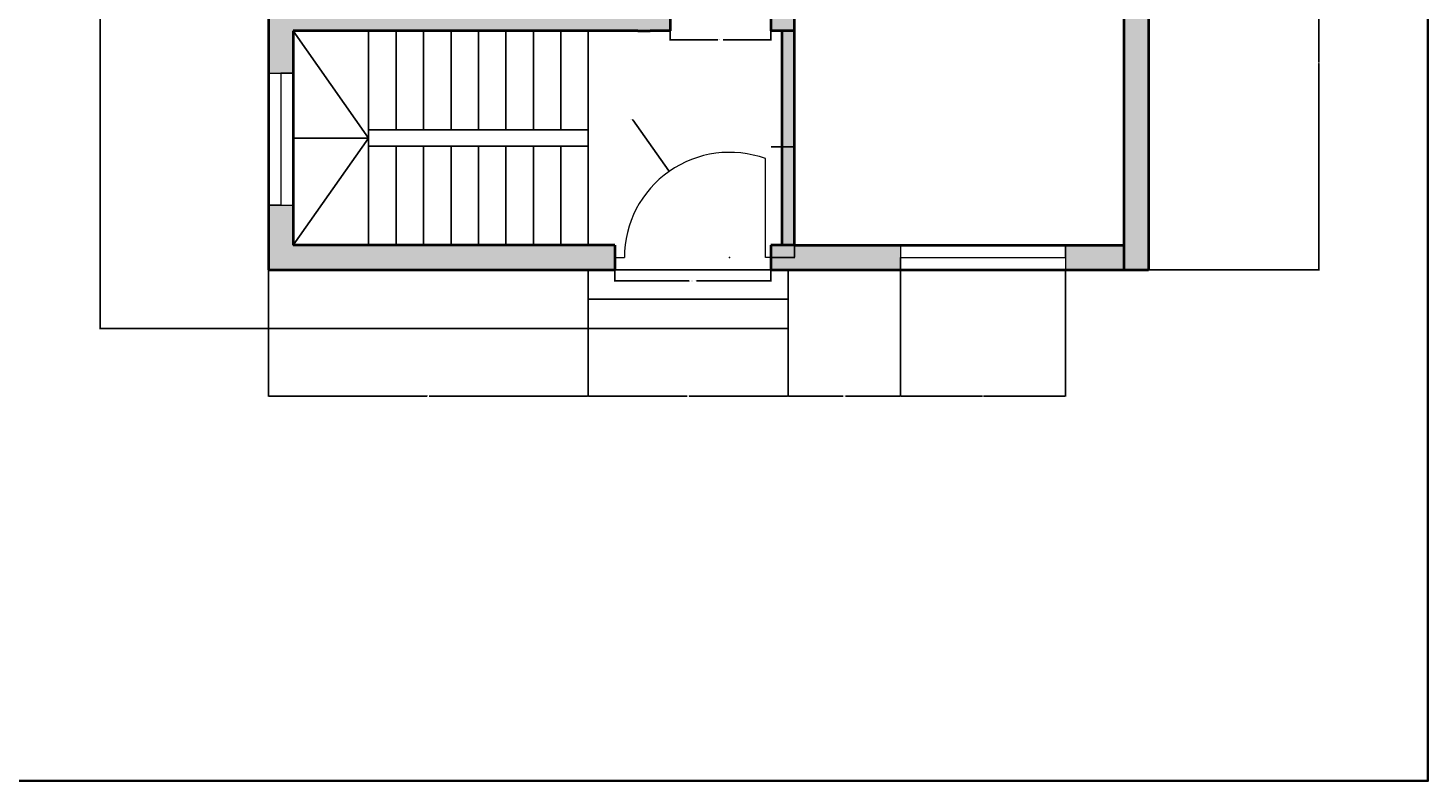
# Model space of a CAD drawing. Units: inches. Extents: x 1441 to 2460, y 1648 to 2683.
# Tile 30 of 35: x 1950 to 2460, y 1648 to 1922. Entities that reach past the tile are written whole.
import ezdxf

# ---------------------------------------------------------------- set-up
doc = ezdxf.new("R2010")
doc.units = ezdxf.units.IN
for name, color, linetype, lineweight in [('A-ANNO-DIMS', 2, 'Continuous', 18), ('A-ANNO-TTLB', 7, 'Continuous', 35), ('A-DOOR', 3, 'Continuous', 20), ('A-FLOR-STRS', 7, 'Continuous', 25), ('A-GLAZ', 4, 'Continuous', 18), ('A-WALL', 7, 'Continuous', 40)]:
    doc.layers.add(name, color=color, linetype=linetype, lineweight=lineweight)
doc.layers.add('A-WALL-PATT', color=251, linetype='Continuous', lineweight=13, true_color=0x636466)
doc.styles.get("Standard").update_dxf_attribs({"font": 'arial.ttf'})
doc.dimstyles.get("Standard").update_dxf_attribs({"dimtxt": 0.18, "dimasz": 0.18, "dimexe": 0.18, "dimexo": 0.0625, "dimgap": 0.09, "dimtad": 0, "dimtih": 1, "dimtoh": 1, "dimdec": 4, "dimzin": 0, "dimdsep": 46, "dimtxsty": 'Standard', "dimcen": 0.09, "dimadec": 0, "dimazin": 0, "dimtfac": 1, "dimtdec": 4, "dimtofl": 0, "dimtmove": 0, "dimatfit": 3, "dimfxl": 1, "dimtolj": 1, "dimtzin": 0, "dimarcsym": 0})

# ---------------------------------------------------------------- blocks, each defined once
blk = doc.blocks.new('DOOR-ENTRY-OUTER')
for p, q in [((54.89, 0), (54.89, 36)), ((0, 0), (1.52, 0)), ((1.52, 0), (3.52, 0)), ((56.89, 0), (54.89, 0))]:
    blk.add_line(p, q)
blk.add_arc((41.82, 0), 38.3, 70.0399, 180)
blk = doc.blocks.new('WIN-48-SASH')
for p, q in [((9, 48), (4.5, 48)), ((4.5, 48), (4.5, 0)), ((4.5, 0), (0, 0))]:
    blk.add_line(p, q)
blk = doc.blocks.new('STAIR-RETURN-PLAN')
for p, q in [((27.5, 39), (0, 78)), ((27.5, 0), (27.5, 78)), ((37.5, 42), (37.5, 78)), ((47.5, 42), (47.5, 78)), ((57.5, 42), (57.5, 78)), ((67.5, 42), (67.5, 78)), ((77.5, 42), (77.5, 78)), ((87.5, 42), (87.5, 78)), ((97.5, 42), (97.5, 78)), ((107.5, 0), (107.5, 78)), ((107.5, 42), (27.5, 42)), ((27.5, 39), (0, 39)), ((0, 39), (27.5, 39)), ((27.5, 39), (0, 0)), ((107.5, 36), (27.5, 36)), ((37.5, 0), (37.5, 36)), ((47.5, 0), (47.5, 36)), ((57.5, 0), (57.5, 36)), ((67.5, 0), (67.5, 36)), ((77.5, 0), (77.5, 36)), ((87.5, 0), (87.5, 36)), ((97.5, 0), (97.5, 36))]:
    blk.add_line(p, q)
blk = doc.blocks.new('*D54')
at = {"layer": 'A-ANNO-DIMS', "color": 0, "lineweight": -2, "transparency": 16777216}
for p, q in [((2164.02, 1838.63), (2164.02, 1829.98)), ((2220.91, 1838.63), (2220.91, 1829.98)), ((2164.2, 1830.16), (2191.07, 1830.16)), ((2220.73, 1830.16), (2193.86, 1830.16))]:
    blk.add_line(p, q, dxfattribs=at)
at = {"layer": 'A-ANNO-DIMS', "color": 0, "transparency": 16777216}
for points in [[(2164.2, 1830.19), (2164.2, 1830.13), (2164.02, 1830.16)], [(2220.73, 1830.19), (2220.73, 1830.13), (2220.91, 1830.16)]]:
    blk.add_solid(points, dxfattribs=at)
at = {"layer": 'Defpoints', "color": 0, "transparency": 16777216}
for p in [(2164.02, 1838.7), (2220.91, 1838.7), (2220.91, 1830.16)]:
    blk.add_point(p, dxfattribs=at)
at = {"layer": 'A-ANNO-DIMS', "color": 0, "transparency": 16777216, "insert": (2192.46, 1830.16), "char_height": 0.18, "attachment_point": 5}
blk.add_mtext('\\A1;ENTRY DOOR 57 TYP.', dxfattribs=at)
blk = doc.blocks.new('*D55')
at = {"layer": 'A-ANNO-DIMS', "color": 0, "lineweight": -2, "transparency": 16777216}
for p, q in [((2220.97, 1878.96), (2229.62, 1878.96)), ((2229.44, 1878.78), (2229.44, 1859.01)), ((2229.44, 1838.88), (2229.44, 1858.65)), ((2220.97, 1838.7), (2229.62, 1838.7))]:
    blk.add_line(p, q, dxfattribs=at)
at = {"layer": 'A-ANNO-DIMS', "color": 0, "transparency": 16777216}
for points in [[(2229.41, 1878.78), (2229.47, 1878.78), (2229.44, 1878.96)], [(2229.41, 1838.88), (2229.47, 1838.88), (2229.44, 1838.7)]]:
    blk.add_solid(points, dxfattribs=at)
at = {"layer": 'Defpoints', "color": 0, "transparency": 16777216}
for p in [(2220.91, 1878.96), (2229.44, 1878.96), (2220.91, 1838.7)]:
    blk.add_point(p, dxfattribs=at)
at = {"layer": 'A-ANNO-DIMS', "color": 0, "transparency": 16777216, "insert": (2229.44, 1858.83), "char_height": 0.18, "attachment_point": 5}
blk.add_mtext('\\A1;40 TYP.', dxfattribs=at)
blk = doc.blocks.new('*D56')
at = {"layer": 'A-ANNO-DIMS', "color": 0, "lineweight": -2, "transparency": 16777216}
for p, q in [((2184.17, 1923.38), (2184.17, 1917.76)), ((2220.88, 1923.38), (2220.88, 1917.76)), ((2184.35, 1917.94), (2201.59, 1917.94)), ((2220.7, 1917.94), (2203.46, 1917.94))]:
    blk.add_line(p, q, dxfattribs=at)
at = {"layer": 'A-ANNO-DIMS', "color": 0, "transparency": 16777216}
for points in [[(2184.35, 1917.97), (2184.35, 1917.91), (2184.17, 1917.94)], [(2220.7, 1917.97), (2220.7, 1917.91), (2220.88, 1917.94)]]:
    blk.add_solid(points, dxfattribs=at)
at = {"layer": 'Defpoints', "color": 0, "transparency": 16777216}
for p in [(2184.17, 1923.45), (2220.88, 1923.45), (2220.88, 1917.94)]:
    blk.add_point(p, dxfattribs=at)
at = {"layer": 'A-ANNO-DIMS', "color": 0, "transparency": 16777216, "insert": (2202.52, 1917.94), "char_height": 0.18, "attachment_point": 5}
blk.add_mtext('\\A1;DOOR 37 TYP.', dxfattribs=at)
blk = doc.blocks.new('*D81')
at = {"layer": 'A-ANNO-DIMS', "color": 0, "lineweight": -2, "transparency": 16777216}
for p, q in [((2037.84, 2298.7), (1976.42, 2298.7)), ((1976.6, 2298.52), (1976.6, 2055.94)), ((1976.6, 1813), (1976.6, 2055.57)), ((2154.24, 1812.82), (1976.42, 1812.82))]:
    blk.add_line(p, q, dxfattribs=at)
at = {"layer": 'A-ANNO-DIMS', "color": 0, "transparency": 16777216}
for points in [[(1976.57, 2298.52), (1976.63, 2298.52), (1976.6, 2298.7)], [(1976.57, 1813), (1976.63, 1813), (1976.6, 1812.82)]]:
    blk.add_solid(points, dxfattribs=at)
at = {"layer": 'Defpoints', "color": 0, "transparency": 16777216}
for p in [(1976.6, 2298.7), (2037.9, 2298.7), (2154.3, 1812.82)]:
    blk.add_point(p, dxfattribs=at)
at = {"layer": 'A-ANNO-DIMS', "color": 0, "transparency": 16777216, "insert": (1976.6, 2055.76), "char_height": 0.18, "attachment_point": 5}
blk.add_mtext('\\A1;485.9', dxfattribs=at)
blk = doc.blocks.new('*D82')
at = {"layer": 'A-ANNO-DIMS', "color": 0, "lineweight": -2, "transparency": 16777216}
for p, q in [((2037.9, 1834.13), (2037.9, 1788.09)), ((2154.3, 1834.13), (2154.3, 1788.09)), ((2038.08, 1788.27), (2095.72, 1788.27)), ((2154.12, 1788.27), (2096.49, 1788.27))]:
    blk.add_line(p, q, dxfattribs=at)
at = {"layer": 'A-ANNO-DIMS', "color": 0, "transparency": 16777216}
for points in [[(2038.08, 1788.3), (2038.08, 1788.24), (2037.9, 1788.27)], [(2154.12, 1788.3), (2154.12, 1788.24), (2154.3, 1788.27)]]:
    blk.add_solid(points, dxfattribs=at)
at = {"layer": 'Defpoints', "color": 0, "transparency": 16777216}
for p in [(2037.9, 1834.2), (2154.3, 1834.2), (2154.3, 1788.27)]:
    blk.add_point(p, dxfattribs=at)
at = {"layer": 'A-ANNO-DIMS', "color": 0, "transparency": 16777216, "insert": (2096.1, 1788.27), "char_height": 0.18, "attachment_point": 5}
blk.add_mtext('\\A1;116.4', dxfattribs=at)
blk = doc.blocks.new('*D83')
at = {"layer": 'A-ANNO-DIMS', "color": 0, "lineweight": -2, "transparency": 16777216}
for p, q in [((2154.3, 1812.75), (2154.3, 1788.09)), ((2227.18, 1812.75), (2227.18, 1788.09)), ((2154.48, 1788.27), (2190.35, 1788.27)), ((2227, 1788.27), (2191.13, 1788.27))]:
    blk.add_line(p, q, dxfattribs=at)
at = {"layer": 'A-ANNO-DIMS', "color": 0, "transparency": 16777216}
for points in [[(2154.48, 1788.3), (2154.48, 1788.24), (2154.3, 1788.27)], [(2227, 1788.3), (2227, 1788.24), (2227.18, 1788.27)]]:
    blk.add_solid(points, dxfattribs=at)
at = {"layer": 'Defpoints', "color": 0, "transparency": 16777216}
for p in [(2154.3, 1812.82), (2227.18, 1812.82), (2227.18, 1788.27)]:
    blk.add_point(p, dxfattribs=at)
at = {"layer": 'A-ANNO-DIMS', "color": 0, "transparency": 16777216, "insert": (2190.74, 1788.27), "char_height": 0.18, "attachment_point": 5}
blk.add_mtext('\\A1;72.87', dxfattribs=at)
blk = doc.blocks.new('*D84')
at = {"layer": 'A-ANNO-DIMS', "color": 0, "lineweight": -2, "transparency": 16777216}
for p, q in [((2268.13, 1834.13), (2268.13, 1788.09)), ((2227.18, 1812.75), (2227.18, 1788.09)), ((2227.36, 1788.27), (2247.26, 1788.27)), ((2267.95, 1788.27), (2248.05, 1788.27))]:
    blk.add_line(p, q, dxfattribs=at)
at = {"layer": 'A-ANNO-DIMS', "color": 0, "transparency": 16777216}
for points in [[(2227.36, 1788.3), (2227.36, 1788.24), (2227.18, 1788.27)], [(2267.95, 1788.3), (2267.95, 1788.24), (2268.13, 1788.27)]]:
    blk.add_solid(points, dxfattribs=at)
at = {"layer": 'Defpoints', "color": 0, "transparency": 16777216}
for p in [(2268.13, 1834.2), (2227.18, 1812.82), (2268.13, 1788.27)]:
    blk.add_point(p, dxfattribs=at)
at = {"layer": 'A-ANNO-DIMS', "color": 0, "transparency": 16777216, "insert": (2247.65, 1788.27), "char_height": 0.18, "attachment_point": 5}
blk.add_mtext('\\A1;40.95', dxfattribs=at)
blk = doc.blocks.new('*D85')
at = {"layer": 'A-ANNO-DIMS', "color": 0, "lineweight": -2, "transparency": 16777216}
for p, q in [((2268.13, 1834.13), (2268.13, 1788.09)), ((2328.13, 1834.13), (2328.13, 1788.09)), ((2268.31, 1788.27), (2297.91, 1788.27)), ((2327.95, 1788.27), (2298.35, 1788.27))]:
    blk.add_line(p, q, dxfattribs=at)
at = {"layer": 'A-ANNO-DIMS', "color": 0, "transparency": 16777216}
for points in [[(2268.31, 1788.3), (2268.31, 1788.24), (2268.13, 1788.27)], [(2327.95, 1788.3), (2327.95, 1788.24), (2328.13, 1788.27)]]:
    blk.add_solid(points, dxfattribs=at)
at = {"layer": 'Defpoints', "color": 0, "transparency": 16777216}
for p in [(2268.13, 1834.2), (2328.13, 1834.2), (2328.13, 1788.27)]:
    blk.add_point(p, dxfattribs=at)
at = {"layer": 'A-ANNO-DIMS', "color": 0, "transparency": 16777216, "insert": (2298.13, 1788.27), "char_height": 0.18, "attachment_point": 5}
blk.add_mtext('\\A1;60', dxfattribs=at)
blk = doc.blocks.new('*D86')
at = {"layer": 'A-ANNO-DIMS', "color": 0, "lineweight": -2, "transparency": 16777216}
for p, q in [((2358.46, 1984.83), (2420.62, 1984.83)), ((2420.44, 1984.65), (2420.44, 1909.69)), ((2420.44, 1834.38), (2420.44, 1909.33)), ((2358.46, 1834.2), (2420.62, 1834.2))]:
    blk.add_line(p, q, dxfattribs=at)
at = {"layer": 'A-ANNO-DIMS', "color": 0, "transparency": 16777216}
for points in [[(2420.41, 1984.65), (2420.47, 1984.65), (2420.44, 1984.83)], [(2420.41, 1834.38), (2420.47, 1834.38), (2420.44, 1834.2)]]:
    blk.add_solid(points, dxfattribs=at)
at = {"layer": 'Defpoints', "color": 0, "transparency": 16777216}
for p in [(2358.4, 1984.83), (2420.44, 1984.83), (2358.4, 1834.2)]:
    blk.add_point(p, dxfattribs=at)
at = {"layer": 'A-ANNO-DIMS', "color": 0, "transparency": 16777216, "insert": (2420.44, 1909.51), "char_height": 0.18, "attachment_point": 5}
blk.add_mtext('\\A1;150.64', dxfattribs=at)
blk = doc.blocks.new('*D128')
at = {"layer": 'A-ANNO-DIMS', "color": 0, "lineweight": -2, "transparency": 16777216}
for p, q in [((2170.49, 1888.88), (2170.67, 1888.88)), ((2170.67, 1888.88), (2183.75, 1870.21)), ((2205.75, 1838.7), (2205.93, 1838.7)), ((2205.84, 1838.61), (2205.84, 1838.79))]:
    blk.add_line(p, q, dxfattribs=at)
at = {"layer": 'A-ANNO-DIMS', "color": 0, "transparency": 16777216}
blk.add_solid([(2183.78, 1870.23), (2183.73, 1870.19), (2183.86, 1870.06)], dxfattribs=at)
at = {"layer": 'Defpoints', "color": 0, "transparency": 16777216}
for p in [(2183.86, 1870.06), (2205.84, 1838.7)]:
    blk.add_point(p, dxfattribs=at)
at = {"layer": 'A-ANNO-DIMS', "color": 0, "transparency": 16777216, "insert": (2170.08, 1888.88), "char_height": 0.18, "attachment_point": 5}
blk.add_mtext('\\A1;R38.3', dxfattribs=at)

msp = doc.modelspace()

# ---------------------------------------------------------------- hatches: boundary and pattern name
at = {"layer": 'A-WALL-PATT'}
h = msp.add_hatch(color=256, dxfattribs=at)
h.dxf.hatch_style = 1
h.paths.add_polyline_path([(2096.524, 2298.6952), (2037.9015, 2298.6952), (2037.9015, 2246.9605), (2046.9015, 2246.9605), (2046.9015, 2289.6952), (2096.524, 2289.6952), (2096.524, 2294.1952)])
h.paths.add_polyline_path([(2144.5933, 2298.6952), (2120.524, 2298.6952), (2120.524, 2289.6952), (2144.5933, 2289.6952), (2144.5933, 2294.1952)])
h.paths.add_polyline_path([(2136.4015, 2289.6952), (2131.9015, 2289.6952), (2131.9015, 2233.0622), (2136.4015, 2233.0622)])
h.paths.add_polyline_path([(2184.8877, 2294.3362), (2184.8877, 2295.2788), (2184.8877, 2298.6952), (2168.5933, 2298.6952), (2168.5933, 2289.6952), (2184.8877, 2289.6952)])
h.paths.add_polyline_path([(2176.9015, 2289.6952), (2172.4015, 2289.6952), (2172.4015, 2199.6952), (2176.9015, 2199.6952)])
h.paths.add_polyline_path([(2229.4015, 2204.637), (2224.9015, 2204.637), (2224.9015, 2199.6952), (2136.4015, 2199.6952), (2136.4015, 2204.637), (2131.9015, 2204.637), (2131.9015, 2195.1952), (2229.4015, 2195.1952)])
h.paths.add_polyline_path([(2229.4015, 2289.6952), (2224.9015, 2289.6952), (2224.9015, 2233.0622), (2229.4015, 2233.0622)])
h.paths.add_polyline_path([(2358.4015, 2298.6952), (2208.8877, 2298.6952), (2208.8877, 2289.6952), (2349.4015, 2289.6952), (2349.4015, 2250.8051), (2358.4015, 2250.8051)])
h.paths.add_polyline_path([(2358.4015, 2202.8051), (2349.4015, 2202.8051), (2349.4015, 2157.6952), (2216.9636, 2157.6952), (2216.9636, 2153.1952), (2224.9015, 2153.1952), (2224.9015, 2058.005), (2229.4015, 2058.005), (2229.4015, 2153.1952), (2349.4015, 2153.1952), (2349.4015, 2124.108), (2358.4015, 2124.108)])
h.paths.add_polyline_path([(2358.4015, 1984.8305), (2349.4015, 1984.8305), (2349.4015, 1834.1952), (2358.4015, 1834.1952)])
h.paths.add_polyline_path([(2358.4015, 2076.108), (2349.4015, 2076.108), (2349.4015, 2008.8305), (2358.4015, 2008.8305)])
h.paths.add_polyline_path([(2349.4015, 2027.1952), (2269.9015, 2027.1952), (2269.9015, 2000.9452), (2274.4015, 2000.9452), (2274.4015, 2022.6952), (2349.4015, 2022.6952)])
h.paths.add_polyline_path([(2269.9015, 2027.1952), (2229.4015, 2027.1952), (2229.4015, 2030.7912), (2224.9015, 2030.7912), (2224.9015, 2022.6952), (2269.9015, 2022.6952)])
h.paths.add_polyline_path([(2349.4015, 1974.6952), (2274.4015, 1974.6952), (2274.4015, 1978.7973), (2269.9015, 1978.7973), (2269.9015, 1974.6952), (2263.8979, 1974.6952), (2263.8979, 1970.1952), (2269.9015, 1970.1952), (2274.4015, 1970.1952), (2349.4015, 1970.1952)])
h.paths.add_polyline_path([(2229.4015, 1974.6952), (2224.9015, 1974.6952), (2224.9015, 1925.6952), (2220.8772, 1925.6952), (2220.8772, 1921.1952), (2229.4015, 1921.1952)])
h.paths.add_polyline_path([(2229.4015, 1921.1952), (2224.9015, 1921.1952), (2224.9015, 1843.1952), (2229.4015, 1843.1952)])
h.paths.add_polyline_path([(2268.1291, 1838.6952), (2268.1291, 1843.1952), (2229.4015, 1843.1952), (2220.91, 1843.1952), (2220.91, 1834.1952), (2227.1771, 1834.1952), (2268.1291, 1834.1952)])
h.paths.add_polyline_path([(2349.4015, 1843.1952), (2328.1291, 1843.1952), (2328.1291, 1834.1952), (2349.4015, 1834.1952)])
h.paths.add_polyline_path([(2046.9015, 1857.7914), (2037.9015, 1857.7914), (2037.9015, 1834.1952), (2164.019, 1834.1952), (2164.019, 1838.6952), (2164.019, 1843.1952), (2046.9015, 1843.1952)])
h.paths.add_polyline_path([(2046.9015, 1959.2399), (2042.4015, 1959.2399), (2037.9015, 1959.2399), (2037.9015, 1905.7914), (2046.9015, 1905.7914), (2046.9015, 1921.1952), (2172.4015, 1921.1952), (2176.9015, 1921.1952), (2184.1657, 1921.1952), (2184.1657, 1925.6952), (2176.9015, 1925.6952), (2172.4015, 1925.6952), (2046.9015, 1925.6952)])
h.paths.add_polyline_path([(2046.9015, 2106.6907), (2037.9015, 2106.6907), (2037.9015, 2019.2399), (2046.9015, 2019.2399)])
h.paths.add_polyline_path([(2176.9015, 2051.6952), (2172.4015, 2051.6952), (2172.4015, 2048.6952), (2172.4015, 1925.6952), (2176.9015, 1925.6952)])
h.paths.add_polyline_path([(2172.4015, 2051.6952), (2145.4015, 2051.6952), (2145.4015, 2048.6952), (2172.4015, 2048.6952)])
h.paths.add_polyline_path([(2172.4015, 2102.6952), (2145.4015, 2102.6952), (2145.4015, 2099.6952), (2154.4015, 2099.6952), (2172.4015, 2099.6952)])
h.paths.add_polyline_path([(2176.9015, 2153.1952), (2179.5767, 2153.1952), (2179.5767, 2157.6952), (2176.9015, 2157.6952), (2176.9015, 2195.1952), (2172.4015, 2195.1952), (2172.4015, 2099.6952), (2176.9015, 2099.6952)])
h.paths.add_polyline_path([(2046.9015, 2198.9605), (2037.9015, 2198.9605), (2037.9015, 2166.6907), (2046.9015, 2166.6907)])

# ---------------------------------------------------------------- linework, layer by layer
at = {"layer": 'A-ANNO-TTLB'}
msp.add_lwpolyline([(1440.5107, 2682.6413), (2460.193, 2682.6413), (2460.193, 1648.08), (1440.5107, 1648.08)], close=True, dxfattribs=at)
at = {"layer": 'A-DOOR'}
msp.add_line((2164.019, 1834.1952), (2164.019, 1838.6952), dxfattribs=at)
at = {"layer": 'A-FLOR-STRS'}
for points in [[(2154.3041, 1834.1952), (2227.1771, 1834.1952), (2227.1771, 1823.5061), (2154.3041, 1823.5061)], [(2154.3041, 1834.1952), (2227.1771, 1834.1952), (2227.1771, 1823.5061), (2154.3041, 1823.5061)], [(2154.3041, 1823.5061), (2227.1771, 1823.5061), (2227.1771, 1812.8171), (2154.3041, 1812.8171)]]:
    msp.add_lwpolyline(points, close=True, dxfattribs=at)
at = {"layer": 'A-GLAZ'}
for p, q in [((2037.9015, 1905.7914), (2046.9015, 1905.7914)), ((2037.9015, 1857.7914), (2046.9015, 1857.7914)), ((2268.1291, 1843.1952), (2268.1291, 1834.1952)), ((2328.1291, 1838.6952), (2328.1291, 1843.1952)), ((2328.1291, 1843.1952), (2328.1291, 1834.1952)), ((2268.1291, 1834.1952), (2268.1291, 1838.6952)), ((2268.1291, 1838.6952), (2268.1291, 1838.6952)), ((2268.1291, 1838.6952), (2328.1291, 1838.6952))]:
    msp.add_line(p, q, dxfattribs=at)
at = {"layer": 'A-WALL'}
for p, q in [((2037.9015, 2298.6952), (2037.9015, 1834.1952)), ((2358.4015, 2298.6952), (2358.4015, 1834.1952)), ((2349.4015, 2153.1952), (2349.4015, 1834.1952)), ((2229.4015, 1974.6952), (2229.4015, 1843.1952)), ((2184.1657, 1925.6952), (2184.1657, 1921.1952)), ((2220.8772, 1925.6952), (2220.8772, 1921.1952)), ((2046.9015, 1921.1952), (2046.9015, 1843.1952)), ((2172.4015, 1921.1952), (2046.9015, 1921.1952)), ((2172.4015, 1921.1952), (2176.9015, 1921.1952)), ((2184.1657, 1921.1952), (2176.9015, 1921.1952)), ((2229.4015, 1921.1952), (2220.8772, 1921.1952)), ((2224.9015, 1921.1952), (2224.9015, 1843.1952)), ((2164.019, 1843.1952), (2046.9015, 1843.1952)), ((2164.019, 1843.1952), (2164.019, 1834.1952)), ((2229.4015, 1843.1952), (2220.91, 1843.1952)), ((2220.91, 1843.1952), (2220.91, 1834.1952)), ((2229.4015, 1843.1952), (2349.4015, 1843.1952)), ((2037.9015, 1834.1952), (2164.019, 1834.1952)), ((2220.91, 1834.1952), (2349.4015, 1834.1952)), ((2349.4015, 1834.1952), (2358.4015, 1834.1952))]:
    msp.add_line(p, q, dxfattribs=at)

# ---------------------------------------------------------------- block references
at = {"layer": 'A-DOOR'}
msp.add_blockref('DOOR-ENTRY-OUTER', (2164.0156, 1838.7), dxfattribs=at)
at = {"layer": 'A-FLOR-STRS'}
msp.add_blockref('STAIR-RETURN-PLAN', (2046.9056, 1843.2), dxfattribs=at)
at = {"layer": 'A-GLAZ'}
msp.add_blockref('WIN-48-SASH', (2037.9056, 1857.7909), dxfattribs=at)

# ---------------------------------------------------------------- dimensions: what is measured, and where the dimension line sits
at = {"layer": 'A-ANNO-DIMS'}
for base, p1, p2, override, picture, middle in [((1976.6039, 2298.6952), (2154.3041, 1812.8171), (2037.9015, 2298.6952), {"dimdec": 1, "dimlfac": 1, "dimrnd": 0, "dimzin": 0, "dimdsep": 46, "dimlunit": 2}, '*D81', (1976.6039, 2055.7561)), ((2420.439, 1984.8305), (2358.4015, 1834.1952), (2358.4015, 1984.8305), {"dimdec": 2, "dimlfac": 1, "dimrnd": 0, "dimzin": 0, "dimdsep": 46, "dimlunit": 2}, '*D86', (2420.439, 1909.5128))]:
    dim = msp.add_linear_dim(base=base, p1=p1, p2=p2, angle=90, dimstyle='Standard', override=override, dxfattribs=at)
    dim.commit()
    dim.dimension.update_dxf_attribs({"geometry": picture, "text_midpoint": middle})
for base, p1, p2, text, picture, middle in [((2220.8772, 1917.9385), (2184.1657, 1923.4452), (2220.8772, 1923.4452), 'DOOR <> TYP.', '*D56', (2202.5215, 1917.9385)), ((2220.91, 1830.1615), (2164.019, 1838.6952), (2220.91, 1838.6952), 'ENTRY DOOR <> TYP.', '*D54', (2192.4645, 1830.1615))]:
    dim = msp.add_linear_dim(base=base, p1=p1, p2=p2, text=text, dimstyle='Standard', override={"dimdec": 0, "dimlfac": 1, "dimrnd": 0, "dimzin": 0, "dimdsep": 46, "dimlunit": 2}, dxfattribs=at)
    dim.commit()
    dim.dimension.update_dxf_attribs({"geometry": picture, "text_midpoint": middle})
dim = msp.add_radius_dim(center=(2205.8355, 1838.6952), mpoint=(2183.8562, 1870.0617), dimstyle='Standard', override={"dimdec": 1, "dimlfac": 1, "dimrnd": 0, "dimzin": 0, "dimdsep": 46, "dimlunit": 2}, dxfattribs=at)
dim.commit()
dim.dimension.update_dxf_attribs({"geometry": '*D128', "text_midpoint": (2170.0788, 1888.8815), "dimtype": 164})
dim = msp.add_linear_dim(base=(2229.4437, 1878.9593), p1=(2220.91, 1838.6952), p2=(2220.91, 1878.9593), angle=90, text='<> TYP.', dimstyle='Standard', override={"dimdec": 0, "dimlfac": 1, "dimrnd": 0, "dimzin": 0, "dimdsep": 46, "dimlunit": 2}, dxfattribs=at)
dim.commit()
dim.dimension.update_dxf_attribs({"geometry": '*D55', "text_midpoint": (2229.4437, 1858.8273)})
for base, p1, p2, override, picture, middle in [((2154.3041, 1788.2671), (2037.9015, 1834.1952), (2154.3041, 1834.1952), {"dimdec": 1, "dimlfac": 1, "dimrnd": 0, "dimzin": 0, "dimdsep": 46, "dimlunit": 2}, '*D82', (2096.1028, 1788.2671)), ((2268.1291, 1788.2671), (2227.1771, 1812.8171), (2268.1291, 1834.1952), {"dimdec": 2, "dimlfac": 1, "dimrnd": 0, "dimzin": 0, "dimdsep": 46, "dimlunit": 2}, '*D84', (2247.6531, 1788.2671)), ((2328.1291, 1788.2671), (2268.1291, 1834.1952), (2328.1291, 1834.1952), {"dimdec": 0, "dimlfac": 1, "dimrnd": 0, "dimzin": 0, "dimdsep": 46, "dimlunit": 2}, '*D85', (2298.1291, 1788.2671)), ((2227.1771, 1788.2671), (2154.3041, 1812.8171), (2227.1771, 1812.8171), {"dimdec": 2, "dimlfac": 1, "dimrnd": 0, "dimzin": 0, "dimdsep": 46, "dimlunit": 2}, '*D83', (2190.7406, 1788.2671))]:
    dim = msp.add_linear_dim(base=base, p1=p1, p2=p2, dimstyle='Standard', override=override, dxfattribs=at)
    dim.commit()
    dim.dimension.update_dxf_attribs({"geometry": picture, "text_midpoint": middle})

doc.saveas('drawing.dxf')
